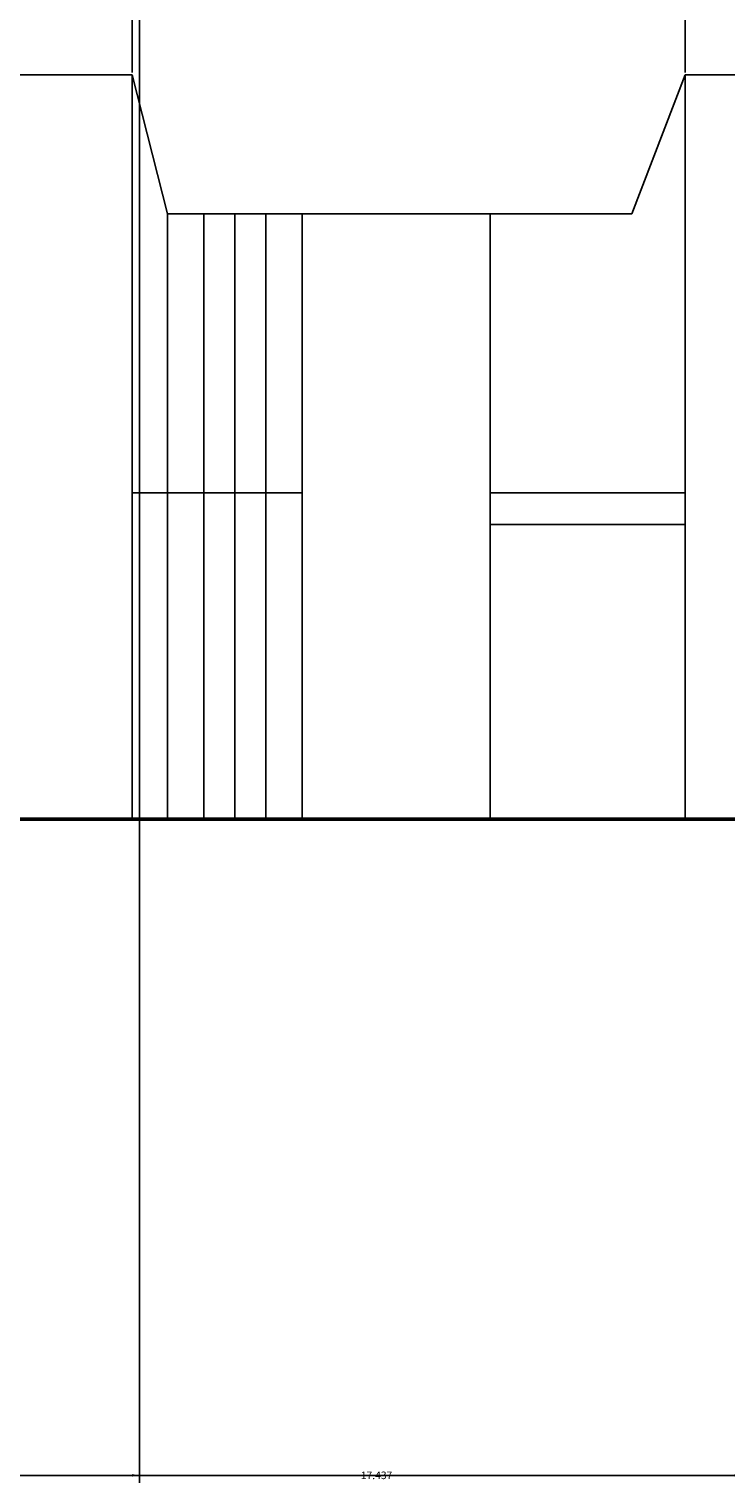
# Model space of a CAD drawing. Units: inches. Extents: x -117 to 121, y -77 to 40.
# Tile 24 of 45: x 55 to 72, y -77 to -43. Entities that reach past the tile are written whole.
import ezdxf

# ---------------------------------------------------------------- set-up
doc = ezdxf.new("R2010")
doc.units = ezdxf.units.IN
doc.header["$MEASUREMENT"] = 0
for name, color, linetype, lineweight in [('A-ANNO-DIMS', 2, 'Continuous', 18), ('A-ELEV', 7, 'Continuous', 25), ('A-ELEV-GRND', 7, 'Continuous', 50)]:
    doc.layers.add(name, color=color, linetype=linetype, lineweight=lineweight)
doc.styles.get("Standard").update_dxf_attribs({"font": 'arial.ttf'})
doc.dimstyles.get("Standard").update_dxf_attribs({"dimtxt": 0.18, "dimasz": 0.18, "dimexe": 0.18, "dimexo": 0.0625, "dimgap": 0.09, "dimtad": 0, "dimtih": 1, "dimtoh": 1, "dimdec": 4, "dimzin": 0, "dimdsep": 46, "dimtxsty": 'Standard', "dimcen": 0.09, "dimadec": 0, "dimazin": 0, "dimtfac": 1, "dimtdec": 4, "dimtofl": 0, "dimtmove": 0, "dimatfit": 3, "dimfxl": 1, "dimtolj": 1, "dimtzin": 0, "dimarcsym": 0})

# ---------------------------------------------------------------- blocks, each defined once
blk = doc.blocks.new('*D7')
at = {"layer": 'A-ANNO-DIMS', "color": 0, "lineweight": -2, "transparency": 16777216}
for p, q in [((-77.763, -61.431), (-77.763, -77.193)), ((90.549, -61.438), (90.549, -77.193)), ((-77.583, -77.013), (6.008, -77.013)), ((90.369, -77.013), (6.778, -77.013))]:
    blk.add_line(p, q, dxfattribs=at)
at = {"layer": 'A-ANNO-DIMS', "color": 0, "transparency": 16777216}
for points in [[(-77.583, -76.983), (-77.583, -77.043), (-77.763, -77.013)], [(90.369, -76.983), (90.369, -77.043), (90.549, -77.013)]]:
    blk.add_solid(points, dxfattribs=at)
at = {"layer": 'Defpoints', "color": 0, "transparency": 16777216}
for p in [(-77.763, -61.369), (90.549, -61.376), (90.549, -77.013)]:
    blk.add_point(p, dxfattribs=at)
at = {"layer": 'A-ANNO-DIMS', "color": 0, "transparency": 16777216, "insert": (6.393, -77.013), "char_height": 0.18, "attachment_point": 5}
blk.add_mtext('\\A1;168.3', dxfattribs=at)
blk = doc.blocks.new('*D28')
at = {"layer": 'A-ANNO-DIMS', "color": 0, "lineweight": -2, "transparency": 16777216}
for p, q in [((54.542, -61.438), (54.542, -77.193)), ((71.979, -61.438), (71.979, -77.193)), ((54.722, -77.013), (62.805, -77.013)), ((71.799, -77.013), (63.716, -77.013))]:
    blk.add_line(p, q, dxfattribs=at)
at = {"layer": 'A-ANNO-DIMS', "color": 0, "transparency": 16777216}
for points in [[(54.722, -76.983), (54.722, -77.043), (54.542, -77.013)], [(71.799, -76.983), (71.799, -77.043), (71.979, -77.013)]]:
    blk.add_solid(points, dxfattribs=at)
at = {"layer": 'Defpoints', "color": 0, "transparency": 16777216}
for p in [(54.542, -61.376), (71.979, -61.376), (71.979, -77.013)]:
    blk.add_point(p, dxfattribs=at)
at = {"layer": 'A-ANNO-DIMS', "color": 0, "transparency": 16777216, "insert": (63.261, -77.013), "char_height": 0.18, "attachment_point": 5}
blk.add_mtext('\\A1;17.437', dxfattribs=at)
blk = doc.blocks.new('*D33')
at = {"layer": 'A-ANNO-DIMS', "color": 0, "lineweight": -2, "transparency": 16777216}
for p, q in [((57.433, -43.571), (57.433, 38.61)), ((70.621, -43.571), (70.621, 38.61)), ((57.613, 38.43), (63.572, 38.43)), ((70.441, 38.43), (64.482, 38.43))]:
    blk.add_line(p, q, dxfattribs=at)
at = {"layer": 'A-ANNO-DIMS', "color": 0, "transparency": 16777216}
for points in [[(57.613, 38.46), (57.613, 38.4), (57.433, 38.43)], [(70.441, 38.46), (70.441, 38.4), (70.621, 38.43)]]:
    blk.add_solid(points, dxfattribs=at)
at = {"layer": 'Defpoints', "color": 0, "transparency": 16777216}
for p in [(70.621, 38.43), (57.433, -43.633), (70.621, -43.633)]:
    blk.add_point(p, dxfattribs=at)
at = {"layer": 'A-ANNO-DIMS', "color": 0, "transparency": 16777216, "insert": (64.027, 38.43), "char_height": 0.18, "attachment_point": 5}
blk.add_mtext('\\A1;13.189', dxfattribs=at)
blk = doc.blocks.new('*D58')
at = {"layer": 'A-ANNO-DIMS', "color": 0, "lineweight": -2, "transparency": 16777216}
for p, q in [((57.61, -7.947), (57.61, -77.193)), ((24.248, -8.105), (24.248, -77.193)), ((24.428, -77.013), (40.467, -77.013)), ((57.43, -77.013), (41.392, -77.013))]:
    blk.add_line(p, q, dxfattribs=at)
at = {"layer": 'A-ANNO-DIMS', "color": 0, "transparency": 16777216}
for points in [[(24.428, -76.983), (24.428, -77.043), (24.248, -77.013)], [(57.43, -76.983), (57.43, -77.043), (57.61, -77.013)]]:
    blk.add_solid(points, dxfattribs=at)
at = {"layer": 'Defpoints', "color": 0, "transparency": 16777216}
for p in [(57.61, -7.885), (24.248, -8.042), (57.61, -77.013)]:
    blk.add_point(p, dxfattribs=at)
at = {"layer": 'A-ANNO-DIMS', "color": 0, "transparency": 16777216, "insert": (40.929, -77.013), "char_height": 0.18, "attachment_point": 5}
blk.add_mtext('\\A1;33.362', dxfattribs=at)

msp = doc.modelspace()

# ---------------------------------------------------------------- linework, layer by layer
at = {"layer": 'A-ELEV'}
for p, q in [((21.9795, -43.6334), (57.4328, -43.6334)), ((57.4328, -43.6334), (57.4328, -61.3756)), ((57.4328, -43.6334), (58.2778, -46.9406)), ((70.6214, -43.6334), (69.3472, -46.9406)), ((70.6214, -61.3756), (70.6214, -43.6334)), ((70.6214, -43.6334), (90.5486, -43.6334)), ((58.2778, -61.3756), (58.2778, -46.9406)), ((58.2778, -46.9406), (69.3472, -46.9406)), ((59.1418, -61.3756), (59.1418, -46.9406)), ((59.8823, -61.3756), (59.8823, -46.9406)), ((60.6229, -61.3756), (60.6229, -46.9406)), ((61.4868, -61.3756), (61.4868, -46.9406)), ((65.9664, -46.9406), (65.9664, -61.3756)), ((57.4328, -53.5899), (61.4868, -53.5899)), ((65.9664, -53.5899), (70.6214, -53.5899)), ((65.9664, -54.35), (70.6214, -54.35))]:
    msp.add_line(p, q, dxfattribs=at)
at = {"layer": 'A-ELEV-GRND'}
msp.add_line((90.5486, -61.3756), (-87.9273, -61.3756), dxfattribs=at)

# ---------------------------------------------------------------- dimensions: what is measured, and where the dimension line sits
at = {"layer": 'A-ANNO-DIMS'}
for base, p1, p2, override, picture, middle in [((70.6214, 38.4297), (57.4328, -43.6334), (70.6214, -43.6334), {"dimdec": 3, "dimlfac": 1, "dimrnd": 0, "dimzin": 0, "dimdsep": 46, "dimlunit": 2}, '*D33', (64.0271, 38.4297)), ((57.6104, -77.0135), (24.2481, -8.0421), (57.6104, -7.8846), {"dimdec": 3, "dimlfac": 1, "dimrnd": 0, "dimzin": 0, "dimdsep": 46, "dimlunit": 2}, '*D58', (40.9293, -77.0135)), ((90.5486, -77.0135), (-77.7631, -61.3689), (90.5486, -61.3756), {"dimdec": 1, "dimlfac": 1, "dimrnd": 0, "dimzin": 0, "dimdsep": 46, "dimlunit": 2}, '*D7', (6.3928, -77.0135)), ((71.9791, -77.0135), (54.5419, -61.3756), (71.9791, -61.3756), {"dimdec": 3, "dimlfac": 1, "dimrnd": 0, "dimzin": 0, "dimdsep": 46, "dimlunit": 2}, '*D28', (63.2605, -77.0135))]:
    dim = msp.add_linear_dim(base=base, p1=p1, p2=p2, dimstyle='Standard', override=override, dxfattribs=at)
    dim.commit()
    dim.dimension.update_dxf_attribs({"geometry": picture, "text_midpoint": middle})

doc.saveas('drawing.dxf')
